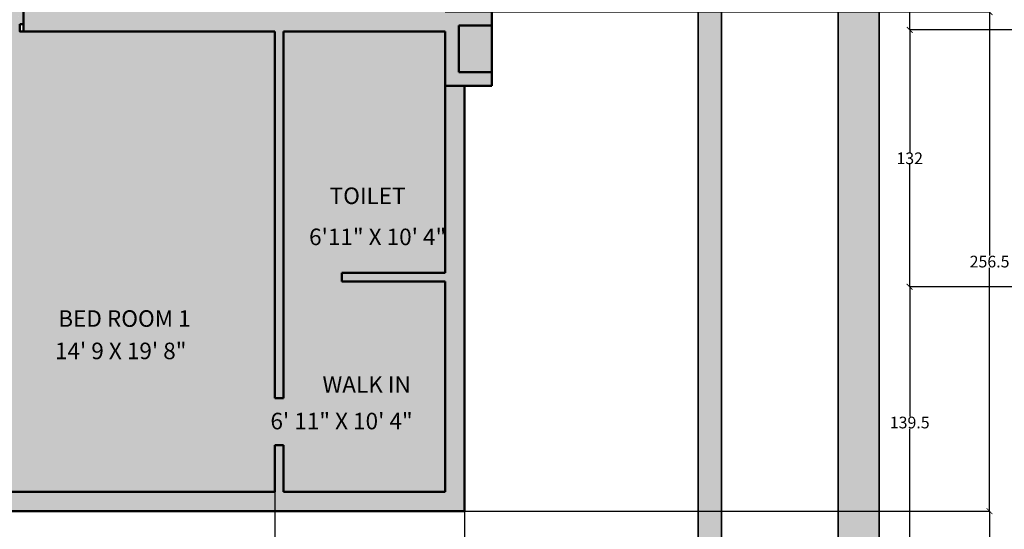
# Model space of a CAD drawing. Units: inches. Extents: x 925 to 2834, y 111 to 1355.
# Tile 6 of 25: x 1490 to 1996, y 376 to 638. Entities that reach past the tile are written whole.
import ezdxf

# ---------------------------------------------------------------- set-up
doc = ezdxf.new("R2010")
doc.units = ezdxf.units.IN
doc.header["$MEASUREMENT"] = 0
for name, color, linetype, lineweight in [('A-ANNO-DIMS', 2, 'Continuous', 18), ('A-ANNO-TTLB', 7, 'Continuous', 35), ('A-AREA-IDEN', 7, 'Continuous', 18), ('A-FLOR-PATT', 252, 'Continuous', 13), ('A-WALL', 7, 'Continuous', 50), ('A-WALL-PATT', 8, 'Continuous', 13)]:
    doc.layers.add(name, color=color, linetype=linetype, lineweight=lineweight)
doc.styles.get("Standard").update_dxf_attribs({"font": 'arial.ttf'})
doc.dimstyles.get("Standard").update_dxf_attribs({"dimtxt": 6, "dimasz": 3, "dimexe": 0.18, "dimexo": 0.0625, "dimgap": 0.09, "dimtad": 0, "dimtih": 1, "dimtoh": 1, "dimdec": 1, "dimzin": 0, "dimdsep": 46, "dimlunit": 3, "dimtxsty": 'Standard', "dimblk": 'ARCHTICK', "dimcen": 0.09, "dimadec": 0, "dimazin": 0, "dimtfac": 1, "dimtdec": 1, "dimtofl": 0, "dimtmove": 0, "dimatfit": 3, "dimfxl": 1, "dimtolj": 1, "dimtzin": 0, "dimarcsym": 0})

# ---------------------------------------------------------------- blocks, each defined once
blk = doc.blocks.new('_ArchTick')
at = {"color": 0, "linetype": 'ByBlock', "const_width": 0.15}
blk.add_lwpolyline([(-0.5, -0.5), (0.5, 0.5)], dxfattribs=at)
blk = doc.blocks.new('*D27')
at = {"layer": 'A-ANNO-DIMS', "color": 0, "lineweight": -2, "transparency": 16777216}
for p, q in [((1621.21, 395.03), (1621.21, 115.18)), ((1434.21, 385.03), (1434.21, 115.18)), ((1434.21, 115.36), (1521.28, 115.36)), ((1621.21, 115.36), (1534.15, 115.36))]:
    blk.add_line(p, q, dxfattribs=at)
at = {"layer": 'Defpoints', "color": 0, "transparency": 16777216}
for p in [(1621.21, 395.09), (1434.21, 385.09), (1621.21, 115.36)]:
    blk.add_point(p, dxfattribs=at)
at = {"layer": 'A-ANNO-DIMS', "color": 0, "lineweight": -2, "transparency": 16777216, "xscale": 3, "yscale": 3, "zscale": 3, "rotation": 180}
blk.add_blockref('_ArchTick', (1434.21, 115.36), dxfattribs=at)
at = {"layer": 'A-ANNO-DIMS', "color": 0, "lineweight": -2, "transparency": 16777216, "xscale": 3, "yscale": 3, "zscale": 3}
blk.add_blockref('_ArchTick', (1621.21, 115.36), dxfattribs=at)
at = {"layer": 'A-ANNO-DIMS', "color": 0, "transparency": 16777216, "insert": (1527.71, 115.36), "char_height": 6, "attachment_point": 5}
blk.add_mtext('\\A1;187', dxfattribs=at)
blk = doc.blocks.new('*D28')
at = {"layer": 'A-ANNO-DIMS', "color": 0, "lineweight": -2, "transparency": 16777216}
for p, q in [((1621.21, 395.03), (1621.21, 115.18)), ((1718.71, 385.03), (1718.71, 115.18)), ((1621.21, 115.36), (1662.06, 115.36)), ((1718.71, 115.36), (1677.87, 115.36))]:
    blk.add_line(p, q, dxfattribs=at)
at = {"layer": 'Defpoints', "color": 0, "transparency": 16777216}
for p in [(1621.21, 395.09), (1718.71, 385.09), (1718.71, 115.36)]:
    blk.add_point(p, dxfattribs=at)
at = {"layer": 'A-ANNO-DIMS', "color": 0, "lineweight": -2, "transparency": 16777216, "xscale": 3, "yscale": 3, "zscale": 3, "rotation": 180}
blk.add_blockref('_ArchTick', (1621.21, 115.36), dxfattribs=at)
at = {"layer": 'A-ANNO-DIMS', "color": 0, "lineweight": -2, "transparency": 16777216, "xscale": 3, "yscale": 3, "zscale": 3}
blk.add_blockref('_ArchTick', (1718.71, 115.36), dxfattribs=at)
at = {"layer": 'A-ANNO-DIMS', "color": 0, "transparency": 16777216, "insert": (1669.96, 115.36), "char_height": 6, "attachment_point": 5}
blk.add_mtext('\\A1;97.5', dxfattribs=at)
blk = doc.blocks.new('*D29')
at = {"layer": 'A-ANNO-DIMS', "color": 0, "lineweight": -2, "transparency": 16777216}
for p, q in [((1718.71, 385.03), (1718.71, 115.18)), ((1838.71, 265.03), (1838.71, 115.18)), ((1718.71, 115.36), (1772.29, 115.36)), ((1838.71, 115.36), (1785.14, 115.36))]:
    blk.add_line(p, q, dxfattribs=at)
at = {"layer": 'Defpoints', "color": 0, "transparency": 16777216}
for p in [(1718.71, 385.09), (1838.71, 265.09), (1838.71, 115.36)]:
    blk.add_point(p, dxfattribs=at)
at = {"layer": 'A-ANNO-DIMS', "color": 0, "lineweight": -2, "transparency": 16777216, "xscale": 3, "yscale": 3, "zscale": 3, "rotation": 180}
blk.add_blockref('_ArchTick', (1718.71, 115.36), dxfattribs=at)
at = {"layer": 'A-ANNO-DIMS', "color": 0, "lineweight": -2, "transparency": 16777216, "xscale": 3, "yscale": 3, "zscale": 3}
blk.add_blockref('_ArchTick', (1838.71, 115.36), dxfattribs=at)
at = {"layer": 'A-ANNO-DIMS', "color": 0, "transparency": 16777216, "insert": (1778.71, 115.36), "char_height": 6, "attachment_point": 5}
blk.add_mtext('\\A1;120', dxfattribs=at)
blk = doc.blocks.new('*D43')
at = {"layer": 'A-ANNO-DIMS', "color": 0, "lineweight": -2, "transparency": 16777216}
for p, q in [((1718.78, 385.09), (1988.62, 385.09)), ((1988.44, 385.09), (1988.44, 328.24)), ((1988.44, 265.09), (1988.44, 321.94)), ((1838.78, 265.09), (1988.62, 265.09))]:
    blk.add_line(p, q, dxfattribs=at)
at = {"layer": 'Defpoints', "color": 0, "transparency": 16777216}
for p in [(1718.71, 385.09), (1988.44, 385.09), (1838.71, 265.09)]:
    blk.add_point(p, dxfattribs=at)
at = {"layer": 'A-ANNO-DIMS', "color": 0, "lineweight": -2, "transparency": 16777216, "xscale": 3, "yscale": 3, "zscale": 3}
for p, rotation in [((1988.44, 385.09), 90), ((1988.44, 265.09), 270)]:
    blk.add_blockref('_ArchTick', p, dxfattribs=dict(at, rotation=rotation))
at = {"layer": 'A-ANNO-DIMS', "color": 0, "transparency": 16777216, "insert": (1988.44, 325.09), "char_height": 6, "attachment_point": 5}
blk.add_mtext('\\A1;120', dxfattribs=at)
blk = doc.blocks.new('*D44')
at = {"layer": 'A-ANNO-DIMS', "color": 0, "lineweight": -2, "transparency": 16777216}
for p, q in [((1708.78, 641.59), (1988.62, 641.59)), ((1988.44, 641.59), (1988.44, 516.49)), ((1988.44, 385.09), (1988.44, 510.19)), ((1718.78, 385.09), (1988.62, 385.09))]:
    blk.add_line(p, q, dxfattribs=at)
at = {"layer": 'Defpoints', "color": 0, "transparency": 16777216}
for p in [(1708.71, 641.59), (1988.44, 641.59), (1718.71, 385.09)]:
    blk.add_point(p, dxfattribs=at)
at = {"layer": 'A-ANNO-DIMS', "color": 0, "lineweight": -2, "transparency": 16777216, "xscale": 3, "yscale": 3, "zscale": 3}
for p, rotation in [((1988.44, 641.59), 90), ((1988.44, 385.09), 270)]:
    blk.add_blockref('_ArchTick', p, dxfattribs=dict(at, rotation=rotation))
at = {"layer": 'A-ANNO-DIMS', "color": 0, "transparency": 16777216, "insert": (1988.44, 513.34), "char_height": 6, "attachment_point": 5}
blk.add_mtext('\\A1;256.5', dxfattribs=at)
blk = doc.blocks.new('*D76')
at = {"layer": 'A-ANNO-DIMS', "color": 0, "lineweight": -2, "transparency": 16777216}
for p, q in [((2124.2, 500.4), (1947.23, 500.4)), ((1947.41, 500.4), (1947.41, 433.8)), ((1947.41, 360.9), (1947.41, 427.49)), ((2124.2, 360.9), (1947.23, 360.9))]:
    blk.add_line(p, q, dxfattribs=at)
at = {"layer": 'Defpoints', "color": 0, "transparency": 16777216}
for p in [(1947.41, 500.4), (2124.26, 500.4), (2124.26, 360.9)]:
    blk.add_point(p, dxfattribs=at)
at = {"layer": 'A-ANNO-DIMS', "color": 0, "lineweight": -2, "transparency": 16777216, "xscale": 3, "yscale": 3, "zscale": 3}
for p, rotation in [((1947.41, 500.4), 90), ((1947.41, 360.9), 270)]:
    blk.add_blockref('_ArchTick', p, dxfattribs=dict(at, rotation=rotation))
at = {"layer": 'A-ANNO-DIMS', "color": 0, "transparency": 16777216, "insert": (1947.41, 430.65), "char_height": 6, "attachment_point": 5}
blk.add_mtext('\\A1;139.5', dxfattribs=at)
blk = doc.blocks.new('*D77')
at = {"layer": 'A-ANNO-DIMS', "color": 0, "lineweight": -2, "transparency": 16777216}
for p, q in [((2134.2, 632.4), (1947.23, 632.4)), ((1947.41, 632.4), (1947.41, 569.55)), ((1947.41, 500.4), (1947.41, 563.24)), ((2124.2, 500.4), (1947.23, 500.4))]:
    blk.add_line(p, q, dxfattribs=at)
at = {"layer": 'Defpoints', "color": 0, "transparency": 16777216}
for p in [(1947.41, 632.4), (2134.26, 632.4), (2124.26, 500.4)]:
    blk.add_point(p, dxfattribs=at)
at = {"layer": 'A-ANNO-DIMS', "color": 0, "lineweight": -2, "transparency": 16777216, "xscale": 3, "yscale": 3, "zscale": 3}
for p, rotation in [((1947.41, 632.4), 90), ((1947.41, 500.4), 270)]:
    blk.add_blockref('_ArchTick', p, dxfattribs=dict(at, rotation=rotation))
at = {"layer": 'A-ANNO-DIMS', "color": 0, "transparency": 16777216, "insert": (1947.41, 566.4), "char_height": 6, "attachment_point": 5}
blk.add_mtext('\\A1;132', dxfattribs=at)
blk = doc.blocks.new('*D78')
at = {"layer": 'A-ANNO-DIMS', "color": 0, "lineweight": -2, "transparency": 16777216}
for p, q in [((2124.2, 808.4), (1947.23, 808.4)), ((1947.41, 808.4), (1947.41, 723.55)), ((1947.41, 632.4), (1947.41, 717.24)), ((2134.2, 632.4), (1947.23, 632.4))]:
    blk.add_line(p, q, dxfattribs=at)
at = {"layer": 'Defpoints', "color": 0, "transparency": 16777216}
for p in [(1947.41, 808.4), (2124.26, 808.4), (2134.26, 632.4)]:
    blk.add_point(p, dxfattribs=at)
at = {"layer": 'A-ANNO-DIMS', "color": 0, "lineweight": -2, "transparency": 16777216, "xscale": 3, "yscale": 3, "zscale": 3}
for p, rotation in [((1947.41, 808.4), 90), ((1947.41, 632.4), 270)]:
    blk.add_blockref('_ArchTick', p, dxfattribs=dict(at, rotation=rotation))
at = {"layer": 'A-ANNO-DIMS', "color": 0, "transparency": 16777216, "insert": (1947.41, 720.4), "char_height": 6, "attachment_point": 5}
blk.add_mtext('\\A1;176', dxfattribs=at)

msp = doc.modelspace()

# ---------------------------------------------------------------- hatches: boundary and pattern name
at = {"layer": 'A-FLOR-PATT', "transparency": 33554605}
h = msp.add_hatch(color=256, dxfattribs=at)
h.dxf.hatch_style = 1
h.paths.add_polyline_path([(1931.688, 1294.5638), (991.7375, 1294.5638), (991.7375, 172.1134), (1931.688, 172.1134)])
h.paths.add_polyline_path([(1910.7128, 1273.5886), (1910.7128, 193.0886), (1012.7128, 193.0886), (1012.7128, 1273.5886)], flags=16)
h.paths.add_polyline_path([(1850.7128, 1213.5886), (1850.7128, 253.0886), (1072.7128, 253.0886), (1072.7128, 1213.5886)], flags=0)
h.paths.add_polyline_path([(1838.7128, 1201.5886), (1838.7128, 265.0886), (1084.7128, 265.0886), (1084.7128, 530.5886), (1084.7128, 1201.5886)], flags=0)
h.paths.add_polyline_path([(1547.6758, 1155.7396), (1547.6758, 1119.115), (1513.0687, 1119.115), (1513.0687, 1155.7396)], flags=0)
h.paths.add_polyline_path([(1600.1067, 1154.9439), (1634.7139, 1154.9439), (1634.7139, 1119.115), (1600.1067, 1119.115)], flags=0)
h.paths.add_polyline_path([(1505.2502, 1144.5358), (1505.2502, 1119.115), (1470.643, 1119.115), (1470.643, 1144.5358)], flags=0)
h.paths.add_polyline_path([(1559.1357, 1141.0962), (1593.7428, 1141.0962), (1593.7428, 1119.115), (1559.1357, 1119.115)], flags=0)
h.paths.add_polyline_path([(1462.8966, 1154.9439), (1462.8966, 1119.115), (1428.2895, 1119.115), (1428.2895, 1154.9439)], flags=0)
h.paths.add_polyline_path([(1642.4603, 1144.5358), (1677.0675, 1144.5358), (1677.0675, 1119.115), (1642.4603, 1119.115)], flags=0)
h.paths.add_polyline_path([(1422.3508, 1141.0962), (1422.3508, 1119.115), (1387.7436, 1119.115), (1387.7436, 1141.0962)], flags=0)
h.paths.add_polyline_path([(1684.8859, 1155.7396), (1719.4931, 1155.7396), (1719.4931, 1119.115), (1684.8859, 1119.115)], flags=0)
h.paths.add_polyline_path([(1718.7128, 1081.5886), (1718.7128, 1050.1249), (1715.7128, 1050.1249), (1715.7128, 1026.1249), (1715.7128, 1002.1249), (1718.7128, 1002.1249), (1730.7128, 1002.1249), (1730.7128, 998.1249), (1730.7128, 990.1249), (1730.7128, 986.1249), (1718.7128, 986.1249), (1718.7128, 893.5886), (1715.3735, 893.5886), (1715.3735, 891.5886), (1713.3735, 891.5886, 0.41421356), (1677.3735, 855.5886), (1713.3735, 855.5886), (1713.3735, 853.5886), (1715.3735, 853.5886), (1715.3735, 851.5886), (1718.7128, 851.5886), (1718.7128, 821.5865), (1734.4655, 821.5865), (1734.3735, 819.5886, -0.41421356), (1712.4415, 793.5886), (1712.4415, 791.5886), (1718.7128, 791.5886), (1718.7128, 717.5886), (1718.7128, 669.5886), (1732.7128, 669.5886), (1732.7128, 665.5886), (1732.7128, 641.5886), (1732.7128, 634.5886), (1732.7128, 610.5886), (1732.7128, 603.5886), (1718.7128, 603.5886), (1718.7128, 385.0886), (1434.2128, 385.0886), (1434.2128, 530.5886), (1410.2128, 530.5886), (1408.2128, 530.5886), (1408.2128, 532.5886, 0.41421356), (1372.2128, 568.5886), (1372.2128, 532.5886), (1370.2128, 532.5886), (1370.2128, 530.5886), (1368.2128, 530.5886), (1282.2128, 530.5886), (1210.2128, 530.5886), (1200.2128, 530.5886), (1200.2128, 542.1915), (1183.2307, 542.1915), (1183.2307, 546.1915), (1200.2128, 546.1915), (1200.2128, 572.1915), (1183.2307, 572.1915), (1183.2307, 576.1915), (1200.2128, 576.1915), (1200.2128, 727.5886), (1210.2128, 727.5886), (1234.2128, 727.5886), (1259.7128, 727.5886), (1259.7128, 775.5886), (1259.7128, 799.5886), (1259.7128, 847.5886), (1259.7128, 993.5872), (1259.7128, 1065.5872), (1259.7128, 1071.5886), (1219.6318, 1071.5886), (1219.6318, 1081.5886), (1084.7128, 1081.5886), (1084.7128, 1119.115), (1256.8974, 1119.115), (1256.8974, 1154.9439), (1291.5046, 1154.9439), (1291.5046, 1119.115), (1256.8974, 1119.115), (1256.6723, 1081.5886), (1293.7128, 1081.5886), (1341.7128, 1081.5886), (1341.7128, 1093.5886), (1347.7128, 1093.5886), (1371.7128, 1093.5886), (1377.7128, 1093.5886), (1377.7128, 1081.5886), (1668.7128, 1081.5886), (1668.7128, 1117.5886), (1675.7128, 1117.5886), (1711.7128, 1117.5886), (1718.7128, 1117.5886)], flags=0)
h.paths.add_polyline_path([(1376.2838, 1155.7396), (1376.2838, 1119.115), (1341.6766, 1119.115), (1341.6766, 1155.7396)], flags=0)
h.paths.add_polyline_path([(1341.7128, 1076.0886), (1293.7128, 1076.0886), (1293.7128, 1071.5886), (1269.7128, 1071.5886), (1269.7128, 1065.5872), (1266.7128, 1065.5872), (1266.7128, 1029.5872), (1265.7128, 1029.5872), (1265.7128, 993.5872), (1269.7128, 993.5872), (1269.7128, 903.5886), (1269.7128, 893.5886), (1269.7128, 847.5886), (1265.2128, 847.5886), (1265.2128, 799.5886), (1269.7128, 799.5886), (1269.7128, 775.5886), (1265.2128, 775.5886), (1265.2128, 727.5886), (1269.7128, 727.5886), (1444.2128, 727.5886), (1444.2128, 717.5886), (1234.2128, 717.5886), (1234.2128, 722.0886), (1210.2128, 722.0886), (1210.2128, 717.5886), (1210.2128, 540.5886), (1210.2128, 536.0886), (1282.2128, 536.0886), (1282.2128, 535.0886), (1210.2128, 535.0886), (1210.2128, 540.5886), (1210.2128, 717.5886), (1210.2128, 723.0886), (1234.2128, 723.0886), (1234.2128, 717.5886), (1444.2128, 717.5886), (1444.2128, 727.5886), (1269.7128, 727.5886), (1264.2128, 727.5886), (1264.2128, 775.5886), (1269.7128, 775.5886), (1269.7128, 799.5886), (1264.2128, 799.5886), (1264.2128, 847.5886), (1269.7128, 847.5886), (1269.7128, 893.5886), (1269.7128, 903.5886), (1269.7128, 993.5872), (1264.7128, 993.5872), (1264.7128, 1029.5872), (1265.7128, 1029.5872), (1265.7128, 1065.5872), (1269.7128, 1065.5872), (1269.7128, 1071.5886), (1293.7128, 1071.5886), (1293.7128, 1077.0886), (1341.7128, 1077.0886)], flags=0)
h.paths.add_polyline_path([(1730.9529, 1141.0962), (1765.5601, 1141.0962), (1765.5601, 1119.115), (1730.9529, 1119.115)], flags=0)
h.paths.add_polyline_path([(1333.8582, 1144.5358), (1333.8582, 1119.115), (1299.251, 1119.115), (1299.251, 1144.5358)], flags=0)
h.paths.add_polyline_path([(1592.7128, 968.5886), (1596.0342, 968.5886), (1602.7128, 968.5886), (1708.7128, 968.5886), (1708.7128, 903.5886), (1602.7128, 903.5886), (1602.7128, 938.5886), (1592.7128, 938.5886), (1592.7128, 903.5886), (1451.7128, 903.5886), (1451.7128, 893.5886), (1511.7128, 893.5886), (1511.7128, 881.5886), (1515.2128, 881.5886), (1518.7128, 881.5886), (1518.7128, 893.5886), (1592.7128, 893.5886), (1592.7128, 799.5886), (1518.7128, 799.5886), (1518.7128, 857.5886), (1511.7128, 857.5886), (1511.7128, 799.5886), (1511.7128, 772.0886), (1521.7128, 772.0886), (1521.7128, 792.5886), (1592.7128, 792.5886), (1592.7128, 727.5886), (1521.7128, 727.5886), (1521.7128, 748.0886), (1511.7128, 748.0886), (1511.7128, 717.5886), (1708.7128, 717.5886), (1714.2128, 717.5886), (1714.2128, 669.5886), (1708.7128, 669.5886), (1708.7128, 641.5886), (1492.2128, 641.5886), (1492.2128, 631.5886), (1621.2128, 631.5886), (1621.2128, 443.0886), (1625.7128, 443.0886), (1625.7128, 503.0886), (1625.7128, 507.5886), (1625.7128, 631.5886), (1708.7128, 631.5886), (1708.7128, 507.5886), (1655.7128, 507.5886), (1655.7128, 503.0886), (1708.7128, 503.0886), (1708.7128, 395.0886), (1625.7128, 395.0886), (1625.7128, 419.0886), (1621.2128, 419.0886), (1621.2128, 395.0886), (1482.2128, 395.0886), (1482.2128, 385.0886), (1434.2128, 385.0886), (1434.2128, 433.0886), (1444.2128, 433.0886), (1444.2128, 631.5886), (1450.2128, 631.5886), (1450.2128, 634.91), (1452.2128, 634.91), (1452.2128, 669.5886), (1454.2128, 669.5886, -0.40021217), (1490.1712, 635.3173), (1492.2128, 635.3173), (1492.2128, 641.5886), (1564.7128, 641.5886), (1564.7128, 677.5886), (1672.7128, 677.5886), (1672.7128, 681.5886), (1564.7128, 681.5886), (1564.7128, 717.5886), (1511.7128, 717.5886), (1511.7128, 748.0886), (1511.7128, 772.0886), (1511.7128, 799.5886), (1511.7128, 857.5886), (1511.8913, 857.5886), (1511.8913, 859.5886), (1515.6201, 859.5886, 0.41421356), (1537.552, 879.5886), (1513.552, 879.5886), (1511.8913, 879.5886), (1511.8913, 881.5886), (1511.7128, 881.5886), (1511.7128, 893.5886), (1451.7128, 893.5886), (1451.7128, 903.5886), (1592.7128, 903.5886), (1592.7128, 938.5886), (1592.7128, 940.5886), (1596.4415, 940.5886, 0.41421356), (1618.3735, 966.5886), (1594.3735, 966.5886), (1592.7128, 966.5886)], flags=0)
h.paths.add_polyline_path([(1377.7128, 903.5886), (1377.7128, 893.5886), (1305.7128, 893.5886), (1305.7128, 903.5886)], flags=0)
h.paths.add_polyline_path([(1708.7128, 821.5886), (1712.0342, 821.5886), (1712.0342, 819.5886), (1710.3735, 819.5886), (1708.7128, 819.5886)], flags=0)
h.paths.add_polyline_path([(1576.7128, 695.1992), (1575.5896, 693.6649), (1575.9687, 694.6994), (1575.4438, 695.1992), (1575.9687, 695.699), (1575.5896, 696.7335)], flags=0)
h.paths.add_polyline_path([(1565.9817, 662.3134), (1565.4568, 661.8136), (1565.8359, 660.7791), (1564.7128, 662.3134), (1565.8359, 663.8477), (1565.4568, 662.8132)], flags=0)
h.paths.add_polyline_path([(1444.2128, 433.0886), (1444.2128, 395.0886), (1482.2128, 395.0886), (1482.2128, 389.0886), (1438.2128, 389.0886), (1438.2128, 391.8608), (1438.2128, 433.0886)], flags=0)
h.paths.add_polyline_path([(1410.2128, 506.5886), (1410.2128, 289.0886), (1108.7128, 289.0886), (1108.7128, 506.5886)], flags=0)
h.paths.add_polyline_path([(1612.3153, 838.3016), (1680.4151, 838.3016), (1680.4151, 851.3131), (1612.3153, 851.3131)], flags=8)
h.paths.add_polyline_path([(1208.3174, 395.0436), (1282.1017, 395.0436), (1282.1017, 408.0552), (1208.3174, 408.0552)], flags=8)
h.paths.add_polyline_path([(1291.8049, 598.7427), (1369.8017, 598.7427), (1369.8017, 611.7542), (1291.8049, 611.7542)], flags=8)
h.paths.add_polyline_path([(1119.679, 917.3022), (1191.0817, 917.3022), (1191.0817, 930.3137), (1119.679, 930.3137)], flags=8)
h.paths.add_polyline_path([(1332.2261, 815.9808), (1410.2258, 815.9808), (1410.2258, 829.001), (1332.2261, 829.001)], flags=8)
h.paths.add_polyline_path([(1390.9013, 955.8158), (1475.4981, 955.8158), (1475.4981, 968.8273), (1390.9013, 968.8273)], flags=8)
h.paths.add_polyline_path([(1620.3436, 998.9325), (1688.4434, 998.9325), (1688.4434, 1011.944), (1620.3436, 1011.944)], flags=8)
h.paths.add_polyline_path([(1620.3436, 914.1039), (1691.7405, 914.1039), (1691.7405, 927.1155), (1620.3436, 927.1155)], flags=8)
h.paths.add_polyline_path([(1521.4542, 816.005), (1589.5569, 816.005), (1589.5569, 829.0253), (1521.4542, 829.0253)], flags=8)
h.paths.add_polyline_path([(1528.524, 740.3497), (1602.3082, 740.3497), (1602.3082, 753.3613), (1528.524, 753.3613)], flags=8)
h.paths.add_polyline_path([(1627.6094, 762.6128), (1702.3091, 762.6128), (1702.3091, 775.6244), (1627.6094, 775.6244)], flags=8)
h.paths.add_polyline_path([(1610.5442, 657.2751), (1684.3284, 657.2751), (1684.3284, 670.2867), (1610.5442, 670.2867)], flags=8)
h.paths.add_polyline_path([(1636.6983, 519.472), (1711.3981, 519.472), (1711.3981, 532.4835), (1636.6983, 532.4835)], flags=8)
h.paths.add_polyline_path([(1616.8577, 424.8539), (1694.8545, 424.8539), (1694.8545, 437.8654), (1616.8577, 437.8654)], flags=8)
h.paths.add_polyline_path([(1506.1456, 460.8838), (1579.9299, 460.8838), (1579.9299, 473.8953), (1506.1456, 473.8953)], flags=8)
h.paths.add_polyline_path([(1624.6119, 784.6011), (1696.9185, 784.6011), (1696.9185, 797.7864), (1624.6119, 797.7864)], flags=8)
h.paths.add_polyline_path([(1606.3732, 854.2194), (1683.3039, 854.2194), (1683.3039, 867.4048), (1606.3732, 867.4048)], flags=8)
h.paths.add_polyline_path([(1127.8008, 940.3581), (1165.1637, 940.3581), (1165.1637, 953.5348), (1127.8008, 953.5348)], flags=8)
h.paths.add_polyline_path([(1620.8657, 1019.4968), (1677.3447, 1019.4968), (1677.3447, 1032.6735), (1620.8657, 1032.6735)], flags=8)
h.paths.add_polyline_path([(1620.8643, 930.1821), (1703.0564, 930.1821), (1703.0564, 943.3675), (1620.8643, 943.3675)], flags=8)
h.paths.add_polyline_path([(1324.5702, 836.8338), (1408.0892, 836.8338), (1408.0892, 850.0191), (1324.5702, 850.0191)], flags=8)
h.paths.add_polyline_path([(1281.6584, 622.8885), (1383.6213, 622.8885), (1383.6213, 636.0739), (1281.6584, 636.0739)], flags=8)
h.paths.add_polyline_path([(1210.6721, 416.7893), (1269.1299, 416.7893), (1269.1299, 429.9747), (1210.6721, 429.9747)], flags=8)
h.paths.add_polyline_path([(1507.8264, 477.4836), (1586.7329, 477.4836), (1586.7329, 490.669), (1507.8264, 490.669)], flags=8)
h.paths.add_polyline_path([(1643.6238, 443.8135), (1696.6696, 443.8135), (1696.6696, 456.5643), (1643.6238, 456.5643)], flags=8)
h.paths.add_polyline_path([(1647.2466, 540.5638), (1693.1825, 540.5638), (1693.1825, 553.7491), (1647.2466, 553.7491)], flags=8)
h.paths.add_polyline_path([(1626.0633, 668.5064), (1673.3174, 668.5064), (1673.3174, 681.6831), (1626.0633, 681.6831)], flags=8)
h.paths.add_polyline_path([(1538.2915, 830.7872), (1567.5942, 830.7872), (1567.5942, 843.5293), (1538.2915, 843.5293)], flags=8)
h.paths.add_polyline_path([(1530.9338, 754.0477), (1559.576, 754.0477), (1559.576, 766.7898), (1530.9338, 766.7898)], flags=8)
h.paths.add_polyline_path([(1351.2461, 979.2309), (1513.8919, 979.2309), (1513.8919, 992.4076), (1351.2461, 992.4076)], flags=8)
at = {"layer": 'A-FLOR-PATT'}
h = msp.add_hatch(color=256, dxfattribs=at)
h.dxf.hatch_style = 1
h.paths.add_polyline_path([(1850.7128, 1213.5886), (1072.7128, 1213.5886), (1072.7128, 253.0886), (1850.7128, 253.0886)])
h.paths.add_polyline_path([(1084.7128, 1201.5886), (1838.7128, 1201.5886), (1838.7128, 265.0886), (1084.7128, 265.0886)], flags=16)
h.paths.add_polyline_path([(1183.2307, 576.1915), (1200.2128, 576.1915), (1200.2128, 727.5886), (1210.2128, 727.5886), (1234.2128, 727.5886), (1259.7128, 727.5886), (1259.7128, 775.5886), (1259.7128, 799.5886), (1259.7128, 847.5886), (1259.7128, 993.5872), (1259.7128, 1065.5872), (1259.7128, 1071.5886), (1219.6318, 1071.5886), (1219.6318, 1081.5886), (1293.7128, 1081.5886), (1341.7128, 1081.5886), (1341.7128, 1093.5886), (1347.7128, 1093.5886), (1347.7128, 1081.5886), (1371.7128, 1081.5886), (1371.7128, 1093.5886), (1377.7128, 1093.5886), (1377.7128, 1081.5886), (1668.7128, 1081.5886), (1668.7128, 1117.5886), (1675.7128, 1117.5886), (1675.7128, 1081.5886), (1711.7128, 1081.5886), (1711.7128, 1117.5886), (1718.7128, 1117.5886), (1718.7128, 1081.5886), (1718.7128, 1050.1249), (1715.7128, 1050.1249), (1715.7128, 1026.1249), (1715.7128, 1002.1249), (1718.7128, 1002.1249), (1730.7128, 1002.1249), (1730.7128, 998.1249), (1730.7128, 990.1249), (1730.7128, 986.1249), (1718.7128, 986.1249), (1718.7128, 893.5886), (1715.3735, 893.5886), (1715.3735, 891.5886), (1713.3735, 891.5886, 0.41421356), (1677.3735, 855.5886), (1713.3735, 855.5886), (1713.3735, 853.5886), (1715.3735, 853.5886), (1715.3735, 851.5886), (1718.7128, 851.5886), (1718.7128, 821.5865), (1734.4655, 821.5865), (1734.3735, 819.5886, -0.41421356), (1712.4415, 793.5886), (1712.4415, 791.5886), (1718.7128, 791.5886), (1718.7128, 717.5886), (1718.7128, 669.5886), (1732.7128, 669.5886), (1732.7128, 665.5886), (1732.7128, 641.5886), (1732.7128, 634.5886), (1732.7128, 610.5886), (1732.7128, 603.5886), (1718.7128, 603.5886), (1718.7128, 385.0886), (1434.2128, 385.0886), (1434.2128, 433.0886), (1434.2128, 530.5886), (1410.2128, 530.5886), (1408.2128, 530.5886), (1408.2128, 532.5886, 0.41421356), (1372.2128, 568.5886), (1372.2128, 532.5886), (1370.2128, 532.5886), (1370.2128, 530.5886), (1368.2128, 530.5886), (1282.2128, 530.5886), (1210.2128, 530.5886), (1200.2128, 530.5886), (1200.2128, 542.1915), (1183.2307, 542.1915), (1183.2307, 546.1915), (1200.2128, 546.1915), (1200.2128, 572.1915), (1183.2307, 572.1915)], flags=0)
h.paths.add_polyline_path([(1210.2128, 717.5886), (1210.2128, 723.0886), (1234.2128, 723.0886), (1234.2128, 717.5886), (1444.2128, 717.5886), (1444.2128, 727.5886), (1269.7128, 727.5886), (1264.2128, 727.5886), (1264.2128, 775.5886), (1269.7128, 775.5886), (1269.7128, 799.5886), (1264.2128, 799.5886), (1264.2128, 847.5886), (1269.7128, 847.5886), (1269.7128, 893.5886), (1269.7128, 903.5886), (1269.7128, 993.5872), (1264.7128, 993.5872), (1264.7128, 1029.5872), (1265.7128, 1029.5872), (1265.7128, 1065.5872), (1269.7128, 1065.5872), (1269.7128, 1071.5886), (1293.7128, 1071.5886), (1293.7128, 1077.0886), (1341.7128, 1077.0886), (1341.7128, 1076.0886), (1293.7128, 1076.0886), (1293.7128, 1071.5886), (1269.7128, 1071.5886), (1269.7128, 1065.5872), (1266.7128, 1065.5872), (1266.7128, 1029.5872), (1265.7128, 1029.5872), (1265.7128, 993.5872), (1269.7128, 993.5872), (1269.7128, 903.5886), (1269.7128, 893.5886), (1269.7128, 847.5886), (1265.2128, 847.5886), (1265.2128, 799.5886), (1269.7128, 799.5886), (1269.7128, 775.5886), (1265.2128, 775.5886), (1265.2128, 727.5886), (1269.7128, 727.5886), (1444.2128, 727.5886), (1444.2128, 717.5886), (1234.2128, 717.5886), (1234.2128, 722.0886), (1210.2128, 722.0886), (1210.2128, 717.5886), (1210.2128, 540.5886), (1210.2128, 536.0886), (1282.2128, 536.0886), (1282.2128, 535.0886), (1210.2128, 535.0886), (1210.2128, 540.5886)], flags=0)
h.paths.add_polyline_path([(1450.2128, 634.91), (1452.2128, 634.91), (1452.2128, 669.5886), (1454.2128, 669.5886, -0.40021217), (1490.1712, 635.3173), (1492.2128, 635.3173), (1492.2128, 641.5886), (1564.7128, 641.5886), (1564.7128, 677.5886), (1672.7128, 677.5886), (1672.7128, 681.5886), (1564.7128, 681.5886), (1564.7128, 717.5886), (1511.7128, 717.5886), (1511.7128, 748.0886), (1511.7128, 772.0886), (1511.7128, 799.5886), (1511.7128, 857.5886), (1511.8913, 857.5886), (1511.8913, 859.5886), (1515.6201, 859.5886, 0.41421356), (1537.552, 879.5886), (1513.552, 879.5886), (1511.8913, 879.5886), (1511.8913, 881.5886), (1511.7128, 881.5886), (1511.7128, 893.5886), (1451.7128, 893.5886), (1451.7128, 903.5886), (1592.7128, 903.5886), (1592.7128, 938.5886), (1592.7128, 940.5886), (1596.4415, 940.5886, 0.41421356), (1618.3735, 966.5886), (1594.3735, 966.5886), (1592.7128, 966.5886), (1592.7128, 968.5886), (1596.0342, 968.5886), (1602.7128, 968.5886), (1708.7128, 968.5886), (1708.7128, 903.5886), (1602.7128, 903.5886), (1602.7128, 938.5886), (1592.7128, 938.5886), (1592.7128, 903.5886), (1451.7128, 903.5886), (1451.7128, 893.5886), (1511.7128, 893.5886), (1511.7128, 881.5886), (1518.7128, 881.5886), (1518.7128, 893.5886), (1592.7128, 893.5886), (1592.7128, 799.5886), (1518.7128, 799.5886), (1518.7128, 857.5886), (1511.7128, 857.5886), (1511.7128, 799.5886), (1511.7128, 772.0886), (1521.7128, 772.0886), (1521.7128, 792.5886), (1592.7128, 792.5886), (1592.7128, 727.5886), (1521.7128, 727.5886), (1521.7128, 748.0886), (1511.7128, 748.0886), (1511.7128, 717.5886), (1708.7128, 717.5886), (1714.2128, 717.5886), (1714.2128, 669.5886), (1708.7128, 669.5886), (1708.7128, 641.5886), (1492.2128, 641.5886), (1492.2128, 631.5886), (1621.2128, 631.5886), (1621.2128, 443.0886), (1625.7128, 443.0886), (1625.7128, 503.0886), (1625.7128, 507.5886), (1625.7128, 631.5886), (1708.7128, 631.5886), (1708.7128, 507.5886), (1655.7128, 507.5886), (1655.7128, 503.0886), (1708.7128, 503.0886), (1708.7128, 395.0886), (1625.7128, 395.0886), (1625.7128, 419.0886), (1621.2128, 419.0886), (1621.2128, 395.0886), (1482.2128, 395.0886), (1482.2128, 389.0886), (1438.2128, 389.0886), (1438.2128, 391.8608), (1438.2128, 433.0886), (1444.2128, 433.0886), (1444.2128, 631.5886), (1450.2128, 631.5886)], flags=0)
h.paths.add_polyline_path([(1444.2128, 433.0886), (1444.2128, 395.0886), (1482.2128, 395.0886), (1482.2128, 391.0886), (1440.2128, 391.0886), (1440.2128, 391.8608), (1440.2128, 433.0886)], flags=0)
h.paths.add_polyline_path([(1305.7128, 893.5886), (1305.7128, 903.5886), (1377.7128, 903.5886), (1377.7128, 893.5886)], flags=0)
h.paths.add_polyline_path([(1564.7128, 662.3134), (1565.8359, 663.8477), (1565.4568, 662.8132), (1565.9817, 662.3134), (1565.4568, 661.8136), (1565.8359, 660.7791)], flags=0)
h.paths.add_polyline_path([(1575.4438, 695.1992), (1575.9687, 695.699), (1575.5896, 696.7335), (1576.7128, 695.1992), (1575.5896, 693.6649), (1575.9687, 694.6994)], flags=0)
h.paths.add_polyline_path([(1708.7128, 821.5886), (1712.0342, 821.5886), (1712.0342, 819.5886), (1710.3735, 819.5886), (1708.7128, 819.5886)], flags=0)
h = msp.add_hatch(color=256, dxfattribs=at)
h.dxf.hatch_style = 1
h.paths.add_polyline_path([(1718.7128, 603.5886), (1708.7128, 603.5886), (1708.7128, 507.5886), (1655.7128, 507.5886), (1655.7128, 503.0886), (1708.7128, 503.0886), (1708.7128, 395.0886), (1625.7128, 395.0886), (1625.7128, 419.0886), (1621.2128, 419.0886), (1621.2128, 395.0886), (1482.2128, 395.0886), (1482.2128, 385.0886), (1718.7128, 385.0886)])
h.paths.add_polyline_path([(1625.7128, 631.5886), (1708.7128, 631.5886), (1708.7128, 603.5886), (1718.7128, 603.5886), (1732.7128, 603.5886), (1732.7128, 610.5886), (1715.7128, 610.5886), (1715.7128, 634.5886), (1732.7128, 634.5886), (1732.7128, 641.5886), (1715.7128, 641.5886), (1715.7128, 665.5886), (1732.7128, 665.5886), (1732.7128, 669.5886), (1708.7128, 669.5886), (1708.7128, 641.5886), (1492.2128, 641.5886), (1492.2128, 631.5886), (1621.2128, 631.5886), (1621.2128, 443.0886), (1625.7128, 443.0886), (1625.7128, 503.0886), (1625.7128, 507.5886)])
h.paths.add_polyline_path([(1718.7128, 851.5886), (1708.7128, 851.5886), (1708.7128, 828.5886), (1602.7128, 828.5886), (1602.7128, 893.5886), (1708.7128, 893.5886), (1718.7128, 893.5886), (1718.7128, 986.1249), (1730.7128, 986.1249), (1730.7128, 990.1249), (1718.7128, 990.1249), (1718.7128, 998.1249), (1730.7128, 998.1249), (1730.7128, 1002.1249), (1718.7128, 1002.1249), (1708.7128, 1002.1249), (1708.7128, 975.5886), (1602.7128, 975.5886), (1602.7128, 1011.5886), (1592.7128, 1011.5886), (1592.7128, 968.5886), (1596.0342, 968.5886), (1602.7128, 968.5886), (1708.7128, 968.5886), (1708.7128, 903.5886), (1602.7128, 903.5886), (1602.7128, 938.5886), (1592.7128, 938.5886), (1592.7128, 903.5886), (1451.7128, 903.5886), (1451.7128, 893.5886), (1511.7128, 893.5886), (1511.7128, 881.5886), (1515.2128, 881.5886), (1518.7128, 881.5886), (1518.7128, 893.5886), (1592.7128, 893.5886), (1592.7128, 799.5886), (1518.7128, 799.5886), (1518.7128, 857.5886), (1511.7128, 857.5886), (1511.7128, 799.5886), (1511.7128, 772.0886), (1521.7128, 772.0886), (1521.7128, 792.5886), (1592.7128, 792.5886), (1592.7128, 727.5886), (1521.7128, 727.5886), (1521.7128, 748.0886), (1511.7128, 748.0886), (1511.7128, 717.5886), (1708.7128, 717.5886), (1718.7128, 717.5886), (1718.7128, 727.5886), (1718.7128, 791.5886), (1708.7128, 791.5886), (1708.7128, 727.5886), (1602.7128, 727.5886), (1602.7128, 821.5886), (1708.7128, 821.5886), (1712.0342, 821.5886), (1718.7128, 821.5886)])
h.paths.add_polyline_path([(1718.7128, 1081.5886), (1718.7128, 1117.5886), (1711.7128, 1117.5886), (1711.7128, 1081.5886), (1675.7128, 1081.5886), (1675.7128, 1117.5886), (1668.7128, 1117.5886), (1668.7128, 1081.5886), (1377.7128, 1081.5886), (1377.7128, 1093.5886), (1371.7128, 1093.5886), (1371.7128, 1081.5886), (1347.7128, 1081.5886), (1347.7128, 1093.5886), (1341.7128, 1093.5886), (1341.7128, 1081.5886), (1341.7128, 1071.5886), (1592.7128, 1071.5886), (1592.7128, 1035.5886), (1602.7128, 1035.5886), (1602.7128, 1071.5886), (1708.7128, 1071.5886), (1708.7128, 1050.1249), (1718.7128, 1050.1249)])
h.paths.add_polyline_path([(1293.7128, 1081.5886), (1219.6318, 1081.5886), (1219.6318, 1071.5886), (1259.7128, 1071.5886), (1259.7128, 1065.5872), (1269.7128, 1065.5872), (1269.7128, 1071.5886), (1293.7128, 1071.5886)])
h.paths.add_polyline_path([(1269.7128, 903.5886), (1269.7128, 993.5872), (1259.7128, 993.5872), (1259.7128, 847.5886), (1269.7128, 847.5886), (1269.7128, 893.5886)])
h.paths.add_polyline_path([(1377.7128, 903.5886), (1305.7128, 903.5886), (1305.7128, 893.5886), (1377.7128, 893.5886)])
h.paths.add_polyline_path([(1444.2128, 727.5886), (1269.7128, 727.5886), (1259.7128, 727.5886), (1234.2128, 727.5886), (1234.2128, 717.5886), (1444.2128, 717.5886)])
h.paths.add_polyline_path([(1269.7128, 799.5886), (1259.7128, 799.5886), (1259.7128, 775.5886), (1269.7128, 775.5886)])
h.paths.add_polyline_path([(1444.2128, 631.5886), (1450.2128, 631.5886), (1450.2128, 634.91), (1450.2128, 641.5886), (1434.2128, 641.5886), (1434.2128, 540.5886), (1410.2128, 540.5886), (1410.2128, 530.5886), (1434.2128, 530.5886), (1434.2128, 433.0886), (1444.2128, 433.0886)])
h.paths.add_polyline_path([(1368.2128, 533.91), (1368.2128, 540.5886), (1282.2128, 540.5886), (1282.2128, 530.5886), (1368.2128, 530.5886)])
h.paths.add_polyline_path([(1210.2128, 717.5886), (1210.2128, 727.5886), (1200.2128, 727.5886), (1200.2128, 576.1915), (1183.2307, 576.1915), (1183.2307, 572.1915), (1200.2128, 572.1915), (1200.2128, 546.1915), (1183.2307, 546.1915), (1183.2307, 542.1915), (1200.2128, 542.1915), (1200.2128, 530.5886), (1210.2128, 530.5886), (1210.2128, 540.5886)])
at = {"layer": 'A-FLOR-PATT', "transparency": 33554605}
h = msp.add_hatch(color=256, dxfattribs=at)
h.dxf.hatch_style = 1
h.paths.add_polyline_path([(1592.7128, 938.5886), (1592.7128, 940.5886), (1596.4415, 940.5886, 0.41421356), (1618.3735, 966.5886), (1594.3735, 966.5886), (1592.7128, 966.5886), (1592.7128, 968.5886), (1592.7128, 1011.5886), (1602.7128, 1011.5886), (1602.7128, 975.5886), (1708.7128, 975.5886), (1708.7128, 1002.1249), (1711.7128, 1002.1249), (1711.7128, 1026.1249), (1711.7128, 1050.1249), (1708.7128, 1050.1249), (1708.7128, 1071.5886), (1602.7128, 1071.5886), (1602.7128, 1035.5886), (1592.7128, 1035.5886), (1592.7128, 1071.5886), (1341.7128, 1071.5886), (1293.7128, 1071.5886), (1269.7128, 1071.5886), (1269.7128, 1065.5872), (1269.7128, 993.5872), (1269.7128, 903.5886), (1269.7128, 893.5886), (1269.7128, 847.5886), (1269.7128, 799.5886), (1269.7128, 775.5886), (1269.7128, 727.5886), (1444.2128, 727.5886), (1444.2128, 717.5886), (1234.2128, 717.5886), (1210.2128, 717.5886), (1210.2128, 540.5886), (1282.2128, 540.5886), (1368.2128, 540.5886), (1368.2128, 533.91), (1370.2128, 533.91), (1370.2128, 568.5886), (1372.2128, 568.5886, -0.40021217), (1408.1712, 534.3173), (1410.2128, 534.3173), (1410.2128, 540.5886), (1434.2128, 540.5886), (1434.2128, 641.5886), (1450.2128, 641.5886), (1450.2128, 634.91), (1452.2128, 634.91), (1452.2128, 669.5886), (1454.2128, 669.5886, -0.40021217), (1490.1712, 635.3173), (1492.2128, 635.3173), (1492.2128, 641.5886), (1564.7128, 641.5886), (1564.7128, 677.5886), (1672.7128, 677.5886), (1672.7128, 681.5886), (1564.7128, 681.5886), (1564.7128, 717.5886), (1511.7128, 717.5886), (1511.7128, 748.0886), (1511.7128, 772.0886), (1511.7128, 799.5886), (1511.7128, 857.5886), (1511.8913, 857.5886), (1511.8913, 859.5886), (1515.6201, 859.5886, 0.41421356), (1537.552, 879.5886), (1513.552, 879.5886), (1511.8913, 879.5886), (1511.8913, 881.5886), (1511.7128, 881.5886), (1511.7128, 893.5886), (1451.7128, 893.5886), (1451.7128, 903.5886), (1592.7128, 903.5886)])
h.paths.add_polyline_path([(1377.7128, 903.5886), (1377.7128, 893.5886), (1305.7128, 893.5886), (1305.7128, 903.5886)], flags=16)
h.paths.add_polyline_path([(1592.7128, 893.5886), (1518.7128, 893.5886), (1518.7128, 881.5865), (1537.6441, 881.5865), (1537.552, 879.5886, -0.41421356), (1515.6201, 859.5886), (1515.6201, 857.5886), (1518.7128, 857.5886), (1518.7128, 799.5886), (1592.7128, 799.5886)], flags=17)
h.paths.add_polyline_path([(1291.8049, 598.7427), (1369.8017, 598.7427), (1369.8017, 611.7542), (1291.8049, 611.7542)], flags=24)
h.paths.add_polyline_path([(1332.2261, 815.9808), (1410.2258, 815.9808), (1410.2258, 829.001), (1332.2261, 829.001)], flags=24)
h.paths.add_polyline_path([(1390.9013, 955.8158), (1475.4981, 955.8158), (1475.4981, 968.8273), (1390.9013, 968.8273)], flags=24)
h.paths.add_polyline_path([(1620.3436, 998.9325), (1688.4434, 998.9325), (1688.4434, 1011.944), (1620.3436, 1011.944)], flags=24)
h.paths.add_polyline_path([(1620.8657, 1019.4968), (1677.3447, 1019.4968), (1677.3447, 1032.6735), (1620.8657, 1032.6735)], flags=24)
h.paths.add_polyline_path([(1324.5702, 836.8338), (1408.0892, 836.8338), (1408.0892, 850.0191), (1324.5702, 850.0191)], flags=24)
h.paths.add_polyline_path([(1281.6584, 622.8885), (1383.6213, 622.8885), (1383.6213, 636.0739), (1281.6584, 636.0739)], flags=24)
h.paths.add_polyline_path([(1626.0633, 668.5064), (1673.3174, 668.5064), (1673.3174, 681.6831), (1626.0633, 681.6831)], flags=25)
h.paths.add_polyline_path([(1351.2461, 979.2309), (1513.8919, 979.2309), (1513.8919, 992.4076), (1351.2461, 992.4076)], flags=24)
h.paths.add_polyline_path([(1521.4542, 816.005), (1589.5569, 816.005), (1589.5569, 829.0253), (1521.4542, 829.0253)], flags=24)
h.paths.add_polyline_path([(1538.2915, 830.7872), (1567.5942, 830.7872), (1567.5942, 843.5293), (1538.2915, 843.5293)], flags=24)
h.paths.add_polyline_path([(1636.6983, 519.472), (1711.3981, 519.472), (1711.3981, 532.4835), (1636.6983, 532.4835)], flags=9)
h.paths.add_polyline_path([(1616.8577, 424.8539), (1694.8545, 424.8539), (1694.8545, 437.8654), (1616.8577, 437.8654)], flags=9)
h.paths.add_polyline_path([(1506.1456, 460.8838), (1579.9299, 460.8838), (1579.9299, 473.8953), (1506.1456, 473.8953)], flags=9)
h.paths.add_polyline_path([(1606.3732, 854.2194), (1683.3039, 854.2194), (1683.3039, 867.4048), (1606.3732, 867.4048)], flags=25)
h.paths.add_polyline_path([(1507.8264, 477.4836), (1586.7329, 477.4836), (1586.7329, 490.669), (1507.8264, 490.669)], flags=9)
h.paths.add_polyline_path([(1643.6238, 443.8135), (1696.6696, 443.8135), (1696.6696, 456.5643), (1643.6238, 456.5643)], flags=9)
h.paths.add_polyline_path([(1647.2466, 540.5638), (1693.1825, 540.5638), (1693.1825, 553.7491), (1647.2466, 553.7491)], flags=25)
h = msp.add_hatch(color=256, dxfattribs=at)
h.dxf.hatch_style = 1
h.paths.add_polyline_path([(1621.2128, 631.5886), (1492.2128, 631.5886), (1490.2128, 631.5886), (1490.2128, 633.5886, 0.41421356), (1454.2128, 669.5886), (1454.2128, 633.5886), (1452.2128, 633.5886), (1452.2128, 631.5886), (1450.2128, 631.5886), (1444.2128, 631.5886), (1444.2128, 395.0886), (1482.2128, 395.0886), (1621.2128, 395.0886), (1621.2128, 419.0886), (1625.7128, 419.0886), (1625.7128, 395.0886), (1708.7128, 395.0886), (1708.7128, 503.0886), (1655.7128, 503.0886), (1655.7128, 507.5886), (1708.7128, 507.5886), (1708.7128, 631.5886), (1625.7128, 631.5886), (1625.7128, 507.5886), (1625.7128, 503.0886), (1625.7128, 443.0886), (1621.2128, 443.0886)])
h.paths.add_polyline_path([(1636.6983, 519.472), (1711.3981, 519.472), (1711.3981, 532.4835), (1636.6983, 532.4835)], flags=9)
h.paths.add_polyline_path([(1616.8577, 424.8539), (1694.8545, 424.8539), (1694.8545, 437.8654), (1616.8577, 437.8654)], flags=24)
h.paths.add_polyline_path([(1506.1456, 460.8838), (1579.9299, 460.8838), (1579.9299, 473.8953), (1506.1456, 473.8953)], flags=24)
h.paths.add_polyline_path([(1507.8264, 477.4836), (1586.7329, 477.4836), (1586.7329, 490.669), (1507.8264, 490.669)], flags=24)
h.paths.add_polyline_path([(1643.6238, 443.8135), (1696.6696, 443.8135), (1696.6696, 456.5643), (1643.6238, 456.5643)], flags=24)
h.paths.add_polyline_path([(1647.2466, 540.5638), (1693.1825, 540.5638), (1693.1825, 553.7491), (1647.2466, 553.7491)], flags=24)
h.paths.add_polyline_path([(1612.3153, 838.3016), (1680.4151, 838.3016), (1680.4151, 851.3131), (1612.3153, 851.3131)], flags=9)
h.paths.add_polyline_path([(1291.8049, 598.7427), (1369.8017, 598.7427), (1369.8017, 611.7542), (1291.8049, 611.7542)], flags=9)
h.paths.add_polyline_path([(1119.679, 917.3022), (1191.0817, 917.3022), (1191.0817, 930.3137), (1119.679, 930.3137)], flags=9)
h.paths.add_polyline_path([(1332.2261, 815.9808), (1410.2258, 815.9808), (1410.2258, 829.001), (1332.2261, 829.001)], flags=9)
h.paths.add_polyline_path([(1390.9013, 955.8158), (1475.4981, 955.8158), (1475.4981, 968.8273), (1390.9013, 968.8273)], flags=9)
h.paths.add_polyline_path([(1620.3436, 998.9325), (1688.4434, 998.9325), (1688.4434, 1011.944), (1620.3436, 1011.944)], flags=9)
h.paths.add_polyline_path([(1620.3436, 914.1039), (1691.7405, 914.1039), (1691.7405, 927.1155), (1620.3436, 927.1155)], flags=9)
h.paths.add_polyline_path([(1521.4542, 816.005), (1589.5569, 816.005), (1589.5569, 829.0253), (1521.4542, 829.0253)], flags=9)
h.paths.add_polyline_path([(1528.524, 740.3497), (1602.3082, 740.3497), (1602.3082, 753.3613), (1528.524, 753.3613)], flags=9)
h.paths.add_polyline_path([(1627.6094, 762.6128), (1702.3091, 762.6128), (1702.3091, 775.6244), (1627.6094, 775.6244)], flags=9)
h.paths.add_polyline_path([(1624.6119, 784.6011), (1696.9185, 784.6011), (1696.9185, 797.7864), (1624.6119, 797.7864)], flags=9)
h.paths.add_polyline_path([(1606.3732, 854.2194), (1683.3039, 854.2194), (1683.3039, 867.4048), (1606.3732, 867.4048)], flags=9)
h.paths.add_polyline_path([(1127.8008, 940.3581), (1165.1637, 940.3581), (1165.1637, 953.5348), (1127.8008, 953.5348)], flags=9)
h.paths.add_polyline_path([(1620.8657, 1019.4968), (1677.3447, 1019.4968), (1677.3447, 1032.6735), (1620.8657, 1032.6735)], flags=9)
h.paths.add_polyline_path([(1620.8643, 930.1821), (1703.0564, 930.1821), (1703.0564, 943.3675), (1620.8643, 943.3675)], flags=9)
h.paths.add_polyline_path([(1324.5702, 836.8338), (1408.0892, 836.8338), (1408.0892, 850.0191), (1324.5702, 850.0191)], flags=9)
h.paths.add_polyline_path([(1281.6584, 622.8885), (1383.6213, 622.8885), (1383.6213, 636.0739), (1281.6584, 636.0739)], flags=9)
h.paths.add_polyline_path([(1626.0633, 668.5064), (1673.3174, 668.5064), (1673.3174, 681.6831), (1626.0633, 681.6831)], flags=9)
h.paths.add_polyline_path([(1538.2915, 830.7872), (1567.5942, 830.7872), (1567.5942, 843.5293), (1538.2915, 843.5293)], flags=9)
h.paths.add_polyline_path([(1530.9338, 754.0477), (1559.576, 754.0477), (1559.576, 766.7898), (1530.9338, 766.7898)], flags=9)
h.paths.add_polyline_path([(1351.2461, 979.2309), (1513.8919, 979.2309), (1513.8919, 992.4076), (1351.2461, 992.4076)], flags=9)
at = {"layer": 'A-WALL-PATT', "transparency": 33554605}
h = msp.add_hatch(color=256, dxfattribs=at)
h.dxf.hatch_style = 1
h.paths.add_polyline_path([(1732.7128, 634.5886), (1715.7128, 634.5886), (1715.7128, 610.5886), (1732.7128, 610.5886)])
h.paths.add_polyline_path([(1732.7128, 665.5886), (1715.7128, 665.5886), (1715.7128, 641.5886), (1732.7128, 641.5886)])
h.paths.add_polyline_path([(1730.7128, 998.1249), (1718.7128, 998.1249), (1718.7128, 990.1249), (1730.7128, 990.1249)])

# ---------------------------------------------------------------- linework, layer by layer
at = {"layer": 'A-ANNO-TTLB'}
for p, q in [((1838.7128, 1201.5886), (1838.7128, 265.0886)), ((1838.7128, 265.0886), (1838.7128, 1081.5886))]:
    msp.add_line(p, q, dxfattribs=at)
for points in [[(991.7375, 172.1134), (1931.688, 172.1134), (1931.688, 1294.5638), (991.7375, 1294.5638)], [(1012.7128, 193.0886), (1910.7128, 193.0886), (1910.7128, 1273.5886), (1012.7128, 1273.5886)], [(1072.7128, 253.0886), (1850.7128, 253.0886), (1850.7128, 1213.5886), (1072.7128, 1213.5886)], [(1084.7128, 265.0886), (1838.7128, 265.0886), (1838.7128, 1201.5886), (1084.7128, 1201.5886)]]:
    msp.add_lwpolyline(points, close=True, dxfattribs=at)
at = {"layer": 'A-WALL'}
for p, q in [((1732.7128, 603.5886), (1732.7128, 669.5886)), ((1492.2128, 631.5886), (1492.2128, 641.5886)), ((1732.7128, 634.5886), (1732.7128, 641.5886)), ((1715.7128, 634.5886), (1732.7128, 634.5886)), ((1715.7128, 634.5886), (1715.7128, 610.5886)), ((1732.7128, 634.5886), (1732.7128, 610.5886)), ((1621.2128, 631.5886), (1492.2128, 631.5886)), ((1621.2128, 631.5886), (1621.2128, 443.0886)), ((1708.7128, 631.5886), (1625.7128, 631.5886)), ((1625.7128, 631.5886), (1625.7128, 507.5886)), ((1708.7128, 631.5886), (1708.7128, 507.5886)), ((1715.7128, 610.5886), (1732.7128, 610.5886)), ((1732.7128, 603.5886), (1732.7128, 610.5886)), ((1708.7128, 603.5886), (1732.7128, 603.5886)), ((1718.7128, 603.5886), (1718.7128, 385.0886)), ((1718.7128, 385.0886), (1718.7128, 603.5886)), ((1718.7128, 603.5886), (1732.7128, 603.5886)), ((1625.7128, 503.0886), (1625.7128, 507.5886)), ((1708.7128, 507.5886), (1655.7128, 507.5886)), ((1655.7128, 503.0886), (1655.7128, 507.5886)), ((1625.7128, 503.0886), (1625.7128, 443.0886)), ((1708.7128, 503.0886), (1655.7128, 503.0886)), ((1708.7128, 503.0886), (1708.7128, 395.0886)), ((1621.2128, 443.0886), (1625.7128, 443.0886)), ((1621.2128, 419.0886), (1625.7128, 419.0886)), ((1621.2128, 419.0886), (1621.2128, 395.0886)), ((1625.7128, 419.0886), (1625.7128, 395.0886)), ((1621.2128, 395.0886), (1444.2128, 395.0886)), ((1708.7128, 395.0886), (1625.7128, 395.0886)), ((1718.7128, 385.0886), (1434.2128, 385.0886)), ((1434.2128, 385.0886), (1714, 385.0886)), ((1714, 385.0886), (1718.7128, 385.0886))]:
    msp.add_line(p, q, dxfattribs=at)
msp.add_lwpolyline([(1490.2128, 635.3173), (1492.2128, 635.3173), (1492.2128, 631.5886), (1490.2128, 631.5886)], close=True, dxfattribs=at)

# ---------------------------------------------------------------- texts
at = {"layer": 'A-AREA-IDEN'}
for s, height, p in [('TOILET', 8.49473, (1649.4442, 542.9062)), ('6\'11" X 10\' 4"', 8.494735, (1638.8669, 521.7855)), ('BED ROOM 1', 8.49473, (1510.0239, 479.826)), ('14\' 9 X 19\' 8"', 8.494735, (1508.3142, 463.1972)), ('WALK IN', 8.49473, (1645.749, 445.9445)), ('6\' 11" X 10\' 4"', 8.494735, (1619.0262, 427.1673))]:
    msp.add_text(s, height=height, dxfattribs=at).set_placement(p)

# ---------------------------------------------------------------- dimensions: what is measured, and where the dimension line sits
at = {"layer": 'A-ANNO-DIMS'}
for base, p1, p2, override, picture, middle in [((1947.408, 808.3964), (2134.258, 632.3964), (2124.258, 808.3964), {"dimdec": 0, "dimlfac": 1, "dimrnd": 0, "dimzin": 0, "dimdsep": 46, "dimlunit": 2}, '*D78', (1947.408, 720.3964)), ((1988.438, 641.5886), (1718.7128, 385.0886), (1708.7128, 641.5886), {"dimdec": 1, "dimlfac": 1, "dimrnd": 0, "dimzin": 0, "dimdsep": 46, "dimlunit": 2}, '*D44', (1988.438, 513.3386)), ((1947.408, 632.3964), (2124.258, 500.3964), (2134.258, 632.3964), {"dimdec": 0, "dimlfac": 1, "dimrnd": 0, "dimzin": 0, "dimdsep": 46, "dimlunit": 2}, '*D77', (1947.408, 566.3964)), ((1947.408, 500.3964), (2124.258, 360.8964), (2124.258, 500.3964), {"dimdec": 1, "dimlfac": 1, "dimrnd": 0, "dimzin": 0, "dimdsep": 46, "dimlunit": 2}, '*D76', (1947.408, 430.6464)), ((1988.438, 385.0886), (1838.7128, 265.0886), (1718.7128, 385.0886), {"dimdec": 0, "dimlfac": 1, "dimrnd": 0, "dimzin": 0, "dimdsep": 46, "dimlunit": 2}, '*D43', (1988.438, 325.0886))]:
    dim = msp.add_linear_dim(base=base, p1=p1, p2=p2, angle=90, dimstyle='Standard', override=override, dxfattribs=at)
    dim.commit()
    dim.dimension.update_dxf_attribs({"geometry": picture, "text_midpoint": middle})
for base, p1, p2, override, picture, middle in [((1621.2128, 115.3634), (1434.2128, 385.0886), (1621.2128, 395.0886), {"dimdec": 0, "dimlfac": 1, "dimrnd": 0, "dimzin": 0, "dimdsep": 46, "dimlunit": 2}, '*D27', (1527.7128, 115.3634)), ((1718.7128, 115.3634), (1621.2128, 395.0886), (1718.7128, 385.0886), {"dimdec": 1, "dimlfac": 1, "dimrnd": 0, "dimzin": 0, "dimdsep": 46, "dimlunit": 2}, '*D28', (1669.9628, 115.3634)), ((1838.7128, 115.3634), (1718.7128, 385.0886), (1838.7128, 265.0886), {"dimdec": 0, "dimlfac": 1, "dimrnd": 0, "dimzin": 0, "dimdsep": 46, "dimlunit": 2}, '*D29', (1778.7128, 115.3634))]:
    dim = msp.add_linear_dim(base=base, p1=p1, p2=p2, dimstyle='Standard', override=override, dxfattribs=at)
    dim.commit()
    dim.dimension.update_dxf_attribs({"geometry": picture, "text_midpoint": middle})

doc.saveas('drawing.dxf')
